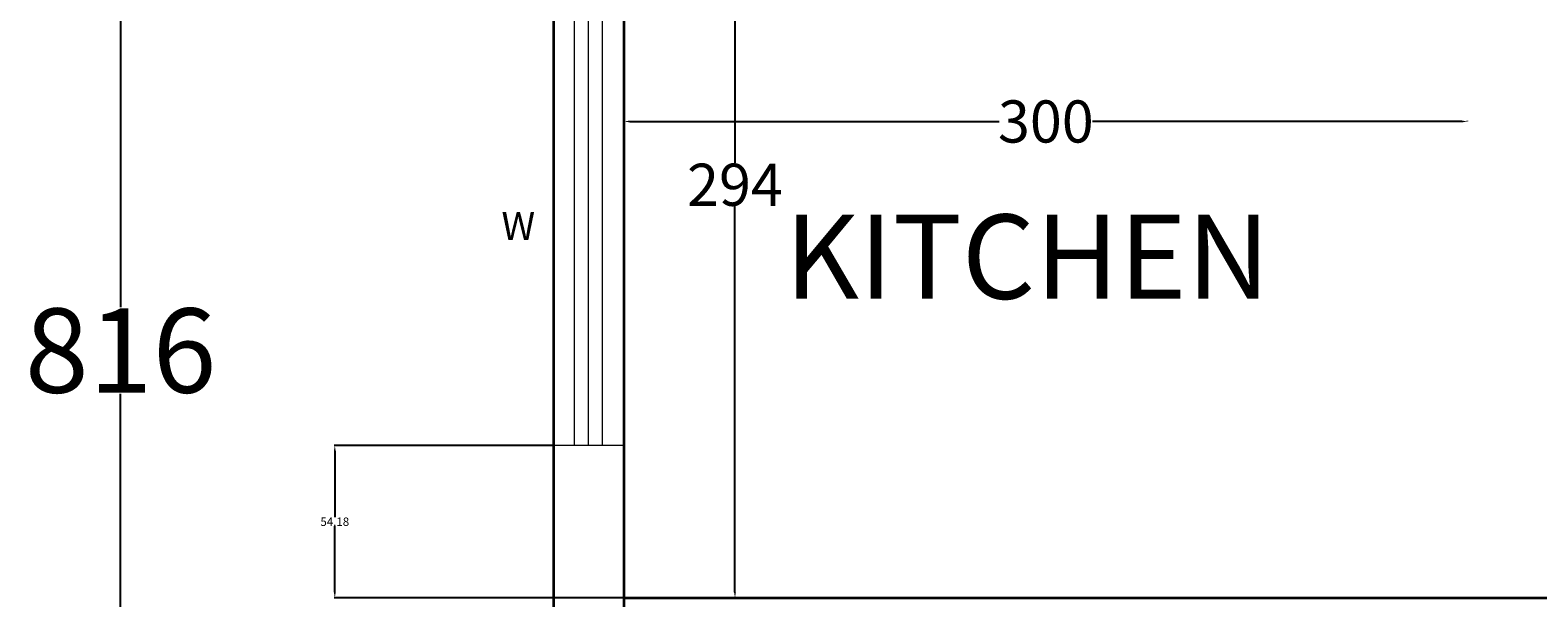
# Model space of a CAD drawing. Units: centimetres. Extents: x -121 to 3851, y -16 to 1180.
# Tile 3 of 16: x -121 to 415, y 384 to 586. Entities that reach past the tile are written whole.
import ezdxf

# ---------------------------------------------------------------- set-up
doc = ezdxf.new("R2010")
doc.units = ezdxf.units.CM
doc.header["$MEASUREMENT"] = 0
for name, color, linetype, lineweight in [('A-ANNO-DIMS', 2, 'Continuous', 18), ('A-ANNO-IDEN', 3, 'Continuous', 13), ('A-AREA-IDEN', 3, 'Continuous', 18), ('A-GLAZ', 4, 'Continuous', 18), ('A-WALL', 7, 'Continuous', 35)]:
    doc.layers.add(name, color=color, linetype=linetype, lineweight=lineweight)
doc.styles.get("Standard").update_dxf_attribs({"font": 'arial.ttf'})
doc.dimstyles.get("Standard").update_dxf_attribs({"dimtxt": 3, "dimasz": 2, "dimexe": 0.18, "dimexo": 0.0625, "dimgap": 0.09, "dimtad": 0, "dimtih": 1, "dimtoh": 1, "dimdec": 0, "dimzin": 0, "dimdsep": 46, "dimtxsty": 'Standard', "dimcen": 0.09, "dimadec": 0, "dimazin": 0, "dimtfac": 1, "dimtdec": 0, "dimtofl": 0, "dimtmove": 0, "dimatfit": 3, "dimfxl": 1, "dimtolj": 1, "dimtzin": 0, "dimarcsym": 0})

# ---------------------------------------------------------------- blocks, each defined once
blk = doc.blocks.new('*D2')
at = {"layer": 'A-ANNO-DIMS', "color": 0, "lineweight": -2, "transparency": 16777216}
for p, q in [((64.98, 880.01), (-89.22, 880.01)), ((-89.04, 878.01), (-89.04, 487.42)), ((-89.04, 66.01), (-89.04, 456.61)), ((64.98, 64.01), (-89.22, 64.01))]:
    blk.add_line(p, q, dxfattribs=at)
at = {"layer": 'A-ANNO-DIMS', "color": 0, "transparency": 16777216}
for points in [[(-89.37, 878.01), (-88.71, 878.01), (-89.04, 880.01)], [(-89.37, 66.01), (-88.71, 66.01), (-89.04, 64.01)]]:
    blk.add_solid(points, dxfattribs=at)
at = {"layer": 'Defpoints', "color": 0, "transparency": 16777216}
for p in [(65.04, 880.01), (-89.04, 64.01), (65.04, 64.01)]:
    blk.add_point(p, dxfattribs=at)
at = {"layer": 'A-ANNO-DIMS', "color": 0, "transparency": 16777216, "insert": (-89.04, 472.01), "char_height": 3, "attachment_point": 5}
blk.add_mtext('\\A1;{\\H10x;816}', dxfattribs=at)
blk = doc.blocks.new('*D5')
at = {"layer": 'A-ANNO-DIMS', "color": 0, "lineweight": -2, "transparency": 16777216}
for p, q in [((196.17, 678.01), (129.29, 678.01)), ((129.47, 676.01), (129.47, 538.76)), ((129.47, 386.01), (129.47, 523.27)), ((196.17, 384.01), (129.29, 384.01))]:
    blk.add_line(p, q, dxfattribs=at)
at = {"layer": 'A-ANNO-DIMS', "color": 0, "transparency": 16777216}
for points in [[(129.13, 676.01), (129.8, 676.01), (129.47, 678.01)], [(129.13, 386.01), (129.8, 386.01), (129.47, 384.01)]]:
    blk.add_solid(points, dxfattribs=at)
at = {"layer": 'Defpoints', "color": 0, "transparency": 16777216}
for p in [(196.23, 678.01), (129.47, 384.01), (196.23, 384.01)]:
    blk.add_point(p, dxfattribs=at)
at = {"layer": 'A-ANNO-DIMS', "color": 0, "transparency": 16777216, "insert": (129.47, 531.01), "char_height": 3, "attachment_point": 5}
blk.add_mtext('\\A1;{\\H5x;294}', dxfattribs=at)
blk = doc.blocks.new('*D6')
at = {"layer": 'A-ANNO-DIMS', "color": 0, "lineweight": -2, "transparency": 16777216}
for p, q in [((90.04, 553.6), (90.04, 553.71)), ((92.04, 553.53), (223.41, 553.53)), ((388.04, 553.53), (256.67, 553.53)), ((390.04, 553.6), (390.04, 553.71))]:
    blk.add_line(p, q, dxfattribs=at)
at = {"layer": 'A-ANNO-DIMS', "color": 0, "transparency": 16777216}
for points in [[(92.04, 553.87), (92.04, 553.2), (90.04, 553.53)], [(388.04, 553.87), (388.04, 553.2), (390.04, 553.53)]]:
    blk.add_solid(points, dxfattribs=at)
at = {"layer": 'Defpoints', "color": 0, "transparency": 16777216}
for p in [(90.04, 553.53), (390.04, 553.53), (390.04, 553.53)]:
    blk.add_point(p, dxfattribs=at)
at = {"layer": 'A-ANNO-DIMS', "color": 0, "transparency": 16777216, "insert": (240.04, 553.53), "char_height": 3, "attachment_point": 5}
blk.add_mtext('\\A1;{\\H5x;300}', dxfattribs=at)
blk = doc.blocks.new('WIN-152CM')
for p, q in [((0, 17.5), (152.19, 17.5)), ((0, 12.5), (152.19, 12.5)), ((0, 7.5), (152.19, 7.5))]:
    blk.add_line(p, q)
blk.add_lwpolyline([(0, 25), (152.19, 25), (152.19, 0), (0, 0)], close=True)
blk = doc.blocks.new('*D43')
at = {"layer": 'A-ANNO-DIMS', "color": 0, "lineweight": -2, "transparency": 16777216}
for p, q in [((64.82, 438.2), (-13.05, 438.2)), ((-12.87, 436.2), (-12.87, 412.73)), ((-12.87, 386.01), (-12.87, 409.48)), ((89.98, 384.01), (-13.05, 384.01))]:
    blk.add_line(p, q, dxfattribs=at)
at = {"layer": 'A-ANNO-DIMS', "color": 0, "transparency": 16777216}
for points in [[(-13.2, 436.2), (-12.53, 436.2), (-12.87, 438.2)], [(-13.2, 386.01), (-12.53, 386.01), (-12.87, 384.01)]]:
    blk.add_solid(points, dxfattribs=at)
at = {"layer": 'Defpoints', "color": 0, "transparency": 16777216}
for p in [(64.88, 438.2), (-12.87, 384.01), (90.04, 384.01)]:
    blk.add_point(p, dxfattribs=at)
at = {"layer": 'A-ANNO-DIMS', "color": 0, "transparency": 16777216, "insert": (-12.87, 411.11), "char_height": 3, "attachment_point": 5}
blk.add_mtext('\\A1;54.18', dxfattribs=at)

msp = doc.modelspace()

# ---------------------------------------------------------------- linework, layer by layer
at = {"layer": 'A-WALL'}
for p, q in [((65.0382, 64.0141), (65.0382, 880.0141)), ((90.0382, 358.0141), (90.0382, 678.0141)), ((90.0382, 384.0141), (595.6084, 384.0141))]:
    msp.add_line(p, q, dxfattribs=at)

# ---------------------------------------------------------------- block references
at = {"layer": 'A-GLAZ', "rotation": 89.99999999999991}
msp.add_blockref('WIN-152CM', (89.8847, 438.1982), dxfattribs=at)

# ---------------------------------------------------------------- texts
at = {"layer": 'A-ANNO-IDEN', "insert": (46.4052, 521.316), "char_height": 10, "attachment_point": 1}
msp.add_mtext_dynamic_manual_height_columns('W', width=55.718495, gutter_width=1, heights=[0], dxfattribs=at)
at = {"layer": 'A-AREA-IDEN', "insert": (147.2034, 520.421), "char_height": 30, "attachment_point": 1}
msp.add_mtext_dynamic_manual_height_columns('KITCHEN', width=147.834071, gutter_width=1, heights=[0], dxfattribs=at)

# ---------------------------------------------------------------- dimensions: what is measured, and where the dimension line sits
at = {"layer": 'A-ANNO-DIMS'}
for base, p1, p2, text, picture, middle in [((-89.041, 64.0141), (65.0382, 880.0141), (65.0382, 64.0141), '{\\H10x;<>}', '*D2', (-89.041, 472.0141)), ((129.4663, 384.0141), (196.2278, 678.0141), (196.2278, 384.0141), '{\\H5x;<>}', '*D5', (129.4663, 531.0141))]:
    dim = msp.add_linear_dim(base=base, p1=p1, p2=p2, angle=90, text=text, dimstyle='Standard', override={"dimclrd": 0, "dimclre": 0, "dimclrt": 0}, dxfattribs=at)
    dim.commit()
    dim.dimension.update_dxf_attribs({"geometry": picture, "text_midpoint": middle})
dim = msp.add_linear_dim(base=(390.0382, 553.5334), p1=(90.0382, 553.5334), p2=(390.0382, 553.5334), text='{\\H5x;<>}', dimstyle='Standard', override={"dimclrd": 0, "dimclre": 0, "dimclrt": 0}, dxfattribs=at)
dim.commit()
dim.dimension.update_dxf_attribs({"geometry": '*D6', "text_midpoint": (240.0382, 553.5334)})
dim = msp.add_linear_dim(base=(-12.8654, 384.0141), p1=(64.8846, 438.1983), p2=(90.0382, 384.0141), angle=90, dimstyle='Standard', override={"dimdec": 2, "dimlfac": 1, "dimrnd": 0, "dimzin": 0, "dimdsep": 46, "dimlunit": 2}, dxfattribs=at)
dim.commit()
dim.dimension.update_dxf_attribs({"geometry": '*D43', "text_midpoint": (-12.8654, 411.1062)})

doc.saveas('drawing.dxf')
